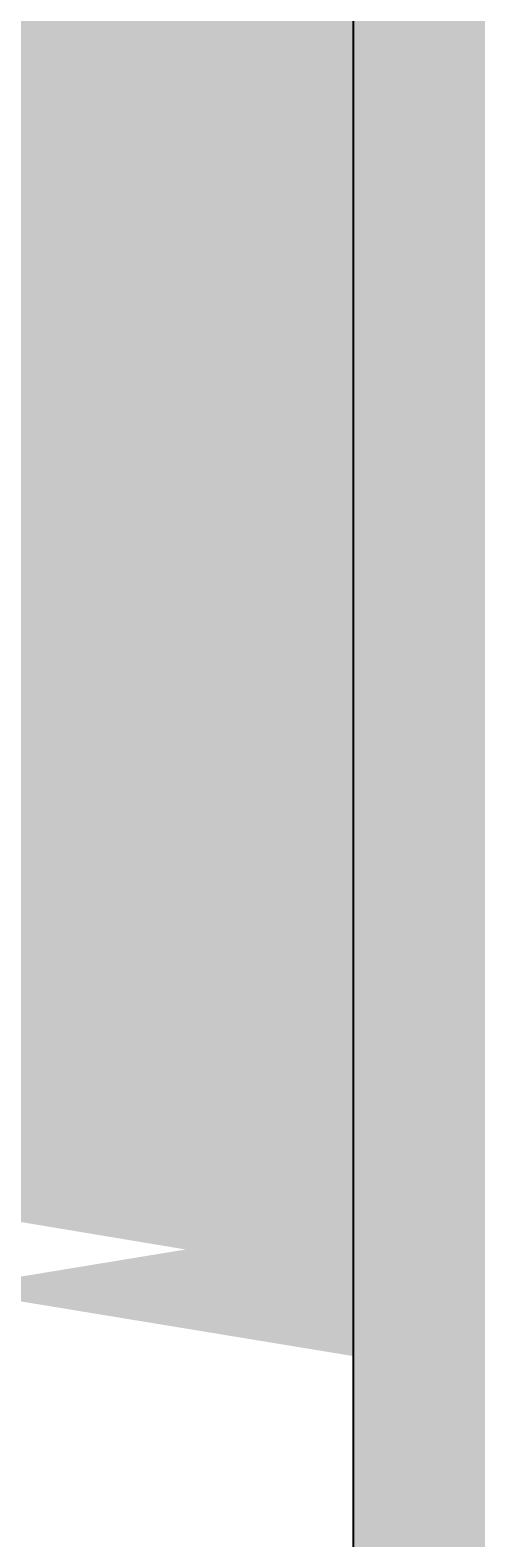
# Model space of a CAD drawing. Units: millimetres. Extents: x -22994 to 29398, y -19990 to 20176.
# Tile 42 of 135: x 190 to 198, y 54 to 78. Entities that reach past the tile are written whole.
import ezdxf
from ezdxf import colors
from ezdxf.entities.mleader import LeaderData, LeaderLine
from ezdxf.math import Vec2, Vec3

# ---------------------------------------------------------------- set-up
doc = ezdxf.new("R2010")
doc.units = ezdxf.units.MM
doc.header["$MEASUREMENT"] = 0
for name, color, linetype, lineweight in [('M-ANNO-TEXT', 7, 'Continuous', 25), ('M-DIMS', 2, 'Continuous', 18), ('M-EQPM', 7, 'Continuous', 25), ('M-EQPM-PATT', 7, 'Continuous', 18)]:
    doc.layers.add(name, color=color, linetype=linetype, lineweight=lineweight)
doc.styles.get("Standard").update_dxf_attribs({"font": 'arial.ttf'})
doc.dimstyles.get("Standard").update_dxf_attribs({"dimtxt": 0.18, "dimasz": 10000, "dimexe": 0.18, "dimexo": 0.0625, "dimgap": 0.09, "dimtad": 0, "dimtih": 1, "dimtoh": 1, "dimdec": 0, "dimzin": 0, "dimdsep": 46, "dimtxsty": 'Standard', "dimcen": 0.09, "dimadec": 0, "dimazin": 0, "dimtfac": 1, "dimtdec": 0, "dimtofl": 0, "dimtmove": 0, "dimatfit": 3, "dimfxl": 1, "dimtolj": 1, "dimtzin": 0, "dimlwd": 30, "dimarcsym": 0})

# ---------------------------------------------------------------- blocks, each defined once
blk = doc.blocks.new('*D2')
at = {"layer": 'Defpoints', "color": 0, "transparency": 16777216}
for p in [(6.677, 10.271), (290.852, 10.271), (290.852, -5.079)]:
    blk.add_point(p, dxfattribs=at)
at = {"layer": 'M-DIMS', "color": 0, "lineweight": -2, "transparency": 16777216}
for p, q in [((6.677, 10.209), (6.677, -5.259)), ((290.852, 10.209), (290.852, -5.259))]:
    blk.add_line(p, q, dxfattribs=at)
at = {"layer": 'M-DIMS', "color": 0, "lineweight": 30, "transparency": 16777216}
for p, q in [((-9993.323, -5.079), (-19993.323, -5.079)), ((10290.852, -5.079), (20290.852, -5.079))]:
    blk.add_line(p, q, dxfattribs=at)
at = {"layer": 'M-DIMS', "color": 0, "transparency": 16777216}
for points in [[(-9993.323, 1661.588), (-9993.323, -1671.745), (6.677, -5.079)], [(10290.852, 1661.588), (10290.852, -1671.745), (290.852, -5.079)]]:
    blk.add_solid(points, dxfattribs=at)
at = {"layer": 'M-DIMS', "color": 0, "transparency": 16777216, "insert": (148.765, -5.079), "char_height": 0.18, "attachment_point": 5}
blk.add_mtext('\\A1;284.2', dxfattribs=at)
blk = doc.blocks.new('*D3')
at = {"layer": 'Defpoints', "color": 0, "transparency": 16777216}
for p in [(110.265, 204.165), (110.265, 176.366), (95.833, 127.967)]:
    blk.add_point(p, dxfattribs=at)
at = {"layer": 'M-DIMS', "color": 0, "lineweight": -2, "transparency": 16777216}
for p, q in [((95.833, 128.03), (95.833, 204.345)), ((110.265, 176.429), (110.265, 204.345))]:
    blk.add_line(p, q, dxfattribs=at)
at = {"layer": 'M-DIMS', "color": 0, "lineweight": 30, "transparency": 16777216}
for p, q in [((-9904.167, 204.165), (-19904.167, 204.165)), ((10110.265, 204.165), (20110.265, 204.165))]:
    blk.add_line(p, q, dxfattribs=at)
at = {"layer": 'M-DIMS', "color": 0, "transparency": 16777216}
for points in [[(-9904.167, 1870.832), (-9904.167, -1462.501), (95.833, 204.165)], [(10110.265, 1870.832), (10110.265, -1462.501), (110.265, 204.165)]]:
    blk.add_solid(points, dxfattribs=at)
at = {"layer": 'M-DIMS', "color": 0, "transparency": 16777216, "insert": (103.049, 204.165), "char_height": 0.18, "attachment_point": 5}
blk.add_mtext('\\A1;14.432', dxfattribs=at)
blk = doc.blocks.new('*D4')
at = {"layer": 'Defpoints', "color": 0, "transparency": 16777216}
for p in [(116.265, 204.165), (110.265, 176.366), (116.265, 176.366)]:
    blk.add_point(p, dxfattribs=at)
at = {"layer": 'M-DIMS', "color": 0, "lineweight": -2, "transparency": 16777216}
for p, q in [((110.265, 176.429), (110.265, 204.345)), ((116.265, 176.429), (116.265, 204.345))]:
    blk.add_line(p, q, dxfattribs=at)
at = {"layer": 'M-DIMS', "color": 0, "lineweight": 30, "transparency": 16777216}
for p, q in [((-9889.735, 204.165), (-19889.735, 204.165)), ((10116.265, 204.165), (20116.265, 204.165))]:
    blk.add_line(p, q, dxfattribs=at)
at = {"layer": 'M-DIMS', "color": 0, "transparency": 16777216}
for points in [[(-9889.735, 1870.832), (-9889.735, -1462.501), (110.265, 204.165)], [(10116.265, 1870.832), (10116.265, -1462.501), (116.265, 204.165)]]:
    blk.add_solid(points, dxfattribs=at)
at = {"layer": 'M-DIMS', "color": 0, "transparency": 16777216, "insert": (113.265, 204.165), "char_height": 0.18, "attachment_point": 5}
blk.add_mtext('\\A1;6', dxfattribs=at)
blk = doc.blocks.new('*D5')
at = {"layer": 'Defpoints', "color": 0, "transparency": 16777216}
for p in [(181.265, 204.165), (116.265, 176.366), (181.265, 176.366)]:
    blk.add_point(p, dxfattribs=at)
at = {"layer": 'M-DIMS', "color": 0, "lineweight": -2, "transparency": 16777216}
for p, q in [((116.265, 176.429), (116.265, 204.345)), ((181.265, 176.429), (181.265, 204.345))]:
    blk.add_line(p, q, dxfattribs=at)
at = {"layer": 'M-DIMS', "color": 0, "lineweight": 30, "transparency": 16777216}
for p, q in [((-9883.735, 204.165), (-19883.735, 204.165)), ((10181.265, 204.165), (20181.265, 204.165))]:
    blk.add_line(p, q, dxfattribs=at)
at = {"layer": 'M-DIMS', "color": 0, "transparency": 16777216}
for points in [[(-9883.735, 1870.832), (-9883.735, -1462.501), (116.265, 204.165)], [(10181.265, 1870.832), (10181.265, -1462.501), (181.265, 204.165)]]:
    blk.add_solid(points, dxfattribs=at)
at = {"layer": 'M-DIMS', "color": 0, "transparency": 16777216, "insert": (148.765, 204.165), "char_height": 0.18, "attachment_point": 5}
blk.add_mtext('\\A1;65', dxfattribs=at)
blk = doc.blocks.new('*D6')
at = {"layer": 'Defpoints', "color": 0, "transparency": 16777216}
for p in [(187.265, 204.165), (181.265, 176.366), (187.265, 176.366)]:
    blk.add_point(p, dxfattribs=at)
at = {"layer": 'M-DIMS', "color": 0, "lineweight": -2, "transparency": 16777216}
for p, q in [((181.265, 176.429), (181.265, 204.345)), ((187.265, 176.429), (187.265, 204.345))]:
    blk.add_line(p, q, dxfattribs=at)
at = {"layer": 'M-DIMS', "color": 0, "lineweight": 30, "transparency": 16777216}
for p, q in [((-9818.735, 204.165), (-19818.735, 204.165)), ((10187.265, 204.165), (20187.265, 204.165))]:
    blk.add_line(p, q, dxfattribs=at)
at = {"layer": 'M-DIMS', "color": 0, "transparency": 16777216}
for points in [[(-9818.735, 1870.832), (-9818.735, -1462.501), (181.265, 204.165)], [(10187.265, 1870.832), (10187.265, -1462.501), (187.265, 204.165)]]:
    blk.add_solid(points, dxfattribs=at)
at = {"layer": 'M-DIMS', "color": 0, "transparency": 16777216, "insert": (184.265, 204.165), "char_height": 0.18, "attachment_point": 5}
blk.add_mtext('\\A1;6', dxfattribs=at)
blk = doc.blocks.new('*D7')
at = {"layer": 'Defpoints', "color": 0, "transparency": 16777216}
for p in [(201.697, 204.165), (187.265, 176.366), (201.697, 127.967)]:
    blk.add_point(p, dxfattribs=at)
at = {"layer": 'M-DIMS', "color": 0, "lineweight": -2, "transparency": 16777216}
for p, q in [((187.265, 176.429), (187.265, 204.345)), ((201.697, 128.03), (201.697, 204.345))]:
    blk.add_line(p, q, dxfattribs=at)
at = {"layer": 'M-DIMS', "color": 0, "lineweight": 30, "transparency": 16777216}
for p, q in [((-9812.735, 204.165), (-19812.735, 204.165)), ((10201.697, 204.165), (20201.697, 204.165))]:
    blk.add_line(p, q, dxfattribs=at)
at = {"layer": 'M-DIMS', "color": 0, "transparency": 16777216}
for points in [[(-9812.735, 1870.832), (-9812.735, -1462.501), (187.265, 204.165)], [(10201.697, 1870.832), (10201.697, -1462.501), (201.697, 204.165)]]:
    blk.add_solid(points, dxfattribs=at)
at = {"layer": 'M-DIMS', "color": 0, "transparency": 16777216, "insert": (194.481, 204.165), "char_height": 0.18, "attachment_point": 5}
blk.add_mtext('\\A1;14.432', dxfattribs=at)
blk = doc.blocks.new('*D8')
at = {"layer": 'Defpoints', "color": 0, "transparency": 16777216}
for p in [(227.648, 204.165), (227.648, 146.73), (201.697, 127.967)]:
    blk.add_point(p, dxfattribs=at)
at = {"layer": 'M-DIMS', "color": 0, "lineweight": -2, "transparency": 16777216}
for p, q in [((201.697, 128.03), (201.697, 204.345)), ((227.648, 146.792), (227.648, 204.345))]:
    blk.add_line(p, q, dxfattribs=at)
at = {"layer": 'M-DIMS', "color": 0, "lineweight": 30, "transparency": 16777216}
for p, q in [((-9798.303, 204.165), (-19798.303, 204.165)), ((10227.648, 204.165), (20227.648, 204.165))]:
    blk.add_line(p, q, dxfattribs=at)
at = {"layer": 'M-DIMS', "color": 0, "transparency": 16777216}
for points in [[(-9798.303, 1870.832), (-9798.303, -1462.501), (201.697, 204.165)], [(10227.648, 1870.832), (10227.648, -1462.501), (227.648, 204.165)]]:
    blk.add_solid(points, dxfattribs=at)
at = {"layer": 'M-DIMS', "color": 0, "transparency": 16777216, "insert": (214.673, 204.165), "char_height": 0.18, "attachment_point": 5}
blk.add_mtext('\\A1;25.95', dxfattribs=at)
blk = doc.blocks.new('*D9')
at = {"layer": 'Defpoints', "color": 0, "transparency": 16777216}
for p in [(187.265, 176.366), (306.202, 176.366), (290.852, 10.271)]:
    blk.add_point(p, dxfattribs=at)
at = {"layer": 'M-DIMS', "color": 0, "lineweight": 30, "transparency": 16777216}
for p, q in [((306.202, 10176.366), (306.202, 20176.366)), ((306.202, -9989.729), (306.202, -19989.729))]:
    blk.add_line(p, q, dxfattribs=at)
at = {"layer": 'M-DIMS', "color": 0, "lineweight": -2, "transparency": 16777216}
for p, q in [((187.327, 176.366), (306.382, 176.366)), ((290.915, 10.271), (306.382, 10.271))]:
    blk.add_line(p, q, dxfattribs=at)
at = {"layer": 'M-DIMS', "color": 0, "transparency": 16777216}
for points in [[(-1360.465, 10176.366), (1972.869, 10176.366), (306.202, 176.366)], [(-1360.465, -9989.729), (1972.869, -9989.729), (306.202, 10.271)]]:
    blk.add_solid(points, dxfattribs=at)
at = {"layer": 'M-DIMS', "color": 0, "transparency": 16777216, "insert": (306.202, 93.319), "char_height": 0.18, "attachment_point": 5}
blk.add_mtext('\\A1;166.1', dxfattribs=at)
blk = doc.blocks.new('*D10')
at = {"layer": 'Defpoints', "color": 0, "transparency": 16777216}
for p in [(125.65, 136.071), (133.346, 136.071), (133.346, -5.079)]:
    blk.add_point(p, dxfattribs=at)
at = {"layer": 'M-DIMS', "color": 0, "lineweight": -2, "transparency": 16777216}
for p, q in [((125.65, 136.009), (125.65, -5.259)), ((133.346, 136.009), (133.346, -5.259))]:
    blk.add_line(p, q, dxfattribs=at)
at = {"layer": 'M-DIMS', "color": 0, "lineweight": 30, "transparency": 16777216}
for p, q in [((-9874.35, -5.079), (-19874.35, -5.079)), ((10133.346, -5.079), (20133.346, -5.079))]:
    blk.add_line(p, q, dxfattribs=at)
at = {"layer": 'M-DIMS', "color": 0, "transparency": 16777216}
for points in [[(-9874.35, 1661.588), (-9874.35, -1671.745), (125.65, -5.079)], [(10133.346, 1661.588), (10133.346, -1671.745), (133.346, -5.079)]]:
    blk.add_solid(points, dxfattribs=at)
at = {"layer": 'M-DIMS', "color": 0, "transparency": 16777216, "insert": (129.498, -5.079), "char_height": 0.18, "attachment_point": 5}
blk.add_mtext('\\A1;7.696', dxfattribs=at)
blk = doc.blocks.new('*D11')
at = {"layer": 'Defpoints', "color": 0, "transparency": 16777216}
for p in [(133.346, 136.071), (135.65, 136.071), (135.65, -5.079)]:
    blk.add_point(p, dxfattribs=at)
at = {"layer": 'M-DIMS', "color": 0, "lineweight": -2, "transparency": 16777216}
for p, q in [((133.346, 136.009), (133.346, -5.259)), ((135.65, 136.009), (135.65, -5.259))]:
    blk.add_line(p, q, dxfattribs=at)
at = {"layer": 'M-DIMS', "color": 0, "lineweight": 30, "transparency": 16777216}
for p, q in [((-9866.654, -5.079), (-19866.654, -5.079)), ((10135.65, -5.079), (20135.65, -5.079))]:
    blk.add_line(p, q, dxfattribs=at)
at = {"layer": 'M-DIMS', "color": 0, "transparency": 16777216}
for points in [[(-9866.654, 1661.588), (-9866.654, -1671.745), (133.346, -5.079)], [(10135.65, 1661.588), (10135.65, -1671.745), (135.65, -5.079)]]:
    blk.add_solid(points, dxfattribs=at)
at = {"layer": 'M-DIMS', "color": 0, "transparency": 16777216, "insert": (134.498, -5.079), "char_height": 0.18, "attachment_point": 5}
blk.add_mtext('\\A1;2.304', dxfattribs=at)
blk = doc.blocks.new('*D12')
at = {"layer": 'Defpoints', "color": 0, "transparency": 16777216}
for p in [(135.65, 136.071), (145.65, 136.071), (145.65, -5.079)]:
    blk.add_point(p, dxfattribs=at)
at = {"layer": 'M-DIMS', "color": 0, "lineweight": -2, "transparency": 16777216}
for p, q in [((135.65, 136.009), (135.65, -5.259)), ((145.65, 136.009), (145.65, -5.259))]:
    blk.add_line(p, q, dxfattribs=at)
at = {"layer": 'M-DIMS', "color": 0, "lineweight": 30, "transparency": 16777216}
for p, q in [((-9864.35, -5.079), (-19864.35, -5.079)), ((10145.65, -5.079), (20145.65, -5.079))]:
    blk.add_line(p, q, dxfattribs=at)
at = {"layer": 'M-DIMS', "color": 0, "transparency": 16777216}
for points in [[(-9864.35, 1661.588), (-9864.35, -1671.745), (135.65, -5.079)], [(10145.65, 1661.588), (10145.65, -1671.745), (145.65, -5.079)]]:
    blk.add_solid(points, dxfattribs=at)
at = {"layer": 'M-DIMS', "color": 0, "transparency": 16777216, "insert": (140.65, -5.079), "char_height": 0.18, "attachment_point": 5}
blk.add_mtext('\\A1;10', dxfattribs=at)
blk = doc.blocks.new('*D13')
at = {"layer": 'Defpoints', "color": 0, "transparency": 16777216}
for p in [(145.65, 136.071), (155.65, 136.071), (155.65, -5.079)]:
    blk.add_point(p, dxfattribs=at)
at = {"layer": 'M-DIMS', "color": 0, "lineweight": -2, "transparency": 16777216}
for p, q in [((145.65, 136.009), (145.65, -5.259)), ((155.65, 136.009), (155.65, -5.259))]:
    blk.add_line(p, q, dxfattribs=at)
at = {"layer": 'M-DIMS', "color": 0, "lineweight": 30, "transparency": 16777216}
for p, q in [((-9854.35, -5.079), (-19854.35, -5.079)), ((10155.65, -5.079), (20155.65, -5.079))]:
    blk.add_line(p, q, dxfattribs=at)
at = {"layer": 'M-DIMS', "color": 0, "transparency": 16777216}
for points in [[(-9854.35, 1661.588), (-9854.35, -1671.745), (145.65, -5.079)], [(10155.65, 1661.588), (10155.65, -1671.745), (155.65, -5.079)]]:
    blk.add_solid(points, dxfattribs=at)
at = {"layer": 'M-DIMS', "color": 0, "transparency": 16777216, "insert": (150.65, -5.079), "char_height": 0.18, "attachment_point": 5}
blk.add_mtext('\\A1;10', dxfattribs=at)
blk = doc.blocks.new('*D14')
at = {"layer": 'Defpoints', "color": 0, "transparency": 16777216}
for p in [(155.65, 136.071), (165.65, 136.071), (165.65, -5.079)]:
    blk.add_point(p, dxfattribs=at)
at = {"layer": 'M-DIMS', "color": 0, "lineweight": -2, "transparency": 16777216}
for p, q in [((155.65, 136.009), (155.65, -5.259)), ((165.65, 136.009), (165.65, -5.259))]:
    blk.add_line(p, q, dxfattribs=at)
at = {"layer": 'M-DIMS', "color": 0, "lineweight": 30, "transparency": 16777216}
for p, q in [((-9844.35, -5.079), (-19844.35, -5.079)), ((10165.65, -5.079), (20165.65, -5.079))]:
    blk.add_line(p, q, dxfattribs=at)
at = {"layer": 'M-DIMS', "color": 0, "transparency": 16777216}
for points in [[(-9844.35, 1661.588), (-9844.35, -1671.745), (155.65, -5.079)], [(10165.65, 1661.588), (10165.65, -1671.745), (165.65, -5.079)]]:
    blk.add_solid(points, dxfattribs=at)
at = {"layer": 'M-DIMS', "color": 0, "transparency": 16777216, "insert": (160.65, -5.079), "char_height": 0.18, "attachment_point": 5}
blk.add_mtext('\\A1;10', dxfattribs=at)
blk = doc.blocks.new('*D15')
at = {"layer": 'Defpoints', "color": 0, "transparency": 16777216}
for p in [(173.346, 154.788), (173.346, 136.071), (306.202, 136.071)]:
    blk.add_point(p, dxfattribs=at)
at = {"layer": 'M-DIMS', "color": 0, "lineweight": 30, "transparency": 16777216}
for p, q in [((306.202, 10154.788), (306.202, 20154.788)), ((306.202, -9863.929), (306.202, -19863.929))]:
    blk.add_line(p, q, dxfattribs=at)
at = {"layer": 'M-DIMS', "color": 0, "lineweight": -2, "transparency": 16777216}
for p, q in [((173.408, 154.788), (306.382, 154.788)), ((173.408, 136.071), (306.382, 136.071))]:
    blk.add_line(p, q, dxfattribs=at)
at = {"layer": 'M-DIMS', "color": 0, "transparency": 16777216}
for points in [[(-1360.465, 10154.788), (1972.869, 10154.788), (306.202, 154.788)], [(-1360.465, -9863.929), (1972.869, -9863.929), (306.202, 136.071)]]:
    blk.add_solid(points, dxfattribs=at)
at = {"layer": 'M-DIMS', "color": 0, "transparency": 16777216, "insert": (306.202, 145.43), "char_height": 0.18, "attachment_point": 5}
blk.add_mtext('\\A1;18.717', dxfattribs=at)
blk = doc.blocks.new('*D16')
at = {"layer": 'Defpoints', "color": 0, "transparency": 16777216}
for p in [(120.17, 204.165), (110.466, 48.035), (120.17, 48.035)]:
    blk.add_point(p, dxfattribs=at)
at = {"layer": 'M-DIMS', "color": 0, "lineweight": -2, "transparency": 16777216}
for p, q in [((110.466, 48.097), (110.466, 204.345)), ((120.17, 48.097), (120.17, 204.345))]:
    blk.add_line(p, q, dxfattribs=at)
at = {"layer": 'M-DIMS', "color": 0, "lineweight": 30, "transparency": 16777216}
for p, q in [((-9889.534, 204.165), (-19889.534, 204.165)), ((10120.17, 204.165), (20120.17, 204.165))]:
    blk.add_line(p, q, dxfattribs=at)
at = {"layer": 'M-DIMS', "color": 0, "transparency": 16777216}
for points in [[(-9889.534, 1870.832), (-9889.534, -1462.501), (110.466, 204.165)], [(10120.17, 1870.832), (10120.17, -1462.501), (120.17, 204.165)]]:
    blk.add_solid(points, dxfattribs=at)
at = {"layer": 'M-DIMS', "color": 0, "transparency": 16777216, "insert": (115.318, 204.165), "char_height": 0.18, "attachment_point": 5}
blk.add_mtext('\\A1;9.704', dxfattribs=at)
blk = doc.blocks.new('*D17')
at = {"layer": 'Defpoints', "color": 0, "transparency": 16777216}
for p in [(126.17, 204.165), (120.17, 48.035), (126.17, 48.035)]:
    blk.add_point(p, dxfattribs=at)
at = {"layer": 'M-DIMS', "color": 0, "lineweight": -2, "transparency": 16777216}
for p, q in [((120.17, 48.097), (120.17, 204.345)), ((126.17, 48.097), (126.17, 204.345))]:
    blk.add_line(p, q, dxfattribs=at)
at = {"layer": 'M-DIMS', "color": 0, "lineweight": 30, "transparency": 16777216}
for p, q in [((-9879.83, 204.165), (-19879.83, 204.165)), ((10126.17, 204.165), (20126.17, 204.165))]:
    blk.add_line(p, q, dxfattribs=at)
at = {"layer": 'M-DIMS', "color": 0, "transparency": 16777216}
for points in [[(-9879.83, 1870.832), (-9879.83, -1462.501), (120.17, 204.165)], [(10126.17, 1870.832), (10126.17, -1462.501), (126.17, 204.165)]]:
    blk.add_solid(points, dxfattribs=at)
at = {"layer": 'M-DIMS', "color": 0, "transparency": 16777216, "insert": (123.17, 204.165), "char_height": 0.18, "attachment_point": 5}
blk.add_mtext('\\A1;6', dxfattribs=at)
blk = doc.blocks.new('*D18')
at = {"layer": 'Defpoints', "color": 0, "transparency": 16777216}
for p in [(132.17, 204.165), (126.17, 48.035), (132.17, 48.035)]:
    blk.add_point(p, dxfattribs=at)
at = {"layer": 'M-DIMS', "color": 0, "lineweight": -2, "transparency": 16777216}
for p, q in [((126.17, 48.097), (126.17, 204.345)), ((132.17, 48.097), (132.17, 204.345))]:
    blk.add_line(p, q, dxfattribs=at)
at = {"layer": 'M-DIMS', "color": 0, "lineweight": 30, "transparency": 16777216}
for p, q in [((-9873.83, 204.165), (-19873.83, 204.165)), ((10132.17, 204.165), (20132.17, 204.165))]:
    blk.add_line(p, q, dxfattribs=at)
at = {"layer": 'M-DIMS', "color": 0, "transparency": 16777216}
for points in [[(-9873.83, 1870.832), (-9873.83, -1462.501), (126.17, 204.165)], [(10132.17, 1870.832), (10132.17, -1462.501), (132.17, 204.165)]]:
    blk.add_solid(points, dxfattribs=at)
at = {"layer": 'M-DIMS', "color": 0, "transparency": 16777216, "insert": (129.17, 204.165), "char_height": 0.18, "attachment_point": 5}
blk.add_mtext('\\A1;6', dxfattribs=at)
blk = doc.blocks.new('*D19')
at = {"layer": 'Defpoints', "color": 0, "transparency": 16777216}
for p in [(138.17, 204.165), (132.17, 48.035), (138.17, 48.035)]:
    blk.add_point(p, dxfattribs=at)
at = {"layer": 'M-DIMS', "color": 0, "lineweight": -2, "transparency": 16777216}
for p, q in [((132.17, 48.097), (132.17, 204.345)), ((138.17, 48.097), (138.17, 204.345))]:
    blk.add_line(p, q, dxfattribs=at)
at = {"layer": 'M-DIMS', "color": 0, "lineweight": 30, "transparency": 16777216}
for p, q in [((-9867.83, 204.165), (-19867.83, 204.165)), ((10138.17, 204.165), (20138.17, 204.165))]:
    blk.add_line(p, q, dxfattribs=at)
at = {"layer": 'M-DIMS', "color": 0, "transparency": 16777216}
for points in [[(-9867.83, 1870.832), (-9867.83, -1462.501), (132.17, 204.165)], [(10138.17, 1870.832), (10138.17, -1462.501), (138.17, 204.165)]]:
    blk.add_solid(points, dxfattribs=at)
at = {"layer": 'M-DIMS', "color": 0, "transparency": 16777216, "insert": (135.17, 204.165), "char_height": 0.18, "attachment_point": 5}
blk.add_mtext('\\A1;6', dxfattribs=at)
blk = doc.blocks.new('*D20')
at = {"layer": 'Defpoints', "color": 0, "transparency": 16777216}
for p in [(144.17, 204.165), (138.17, 48.035), (144.17, 48.035)]:
    blk.add_point(p, dxfattribs=at)
at = {"layer": 'M-DIMS', "color": 0, "lineweight": -2, "transparency": 16777216}
for p, q in [((138.17, 48.097), (138.17, 204.345)), ((144.17, 48.097), (144.17, 204.345))]:
    blk.add_line(p, q, dxfattribs=at)
at = {"layer": 'M-DIMS', "color": 0, "lineweight": 30, "transparency": 16777216}
for p, q in [((-9861.83, 204.165), (-19861.83, 204.165)), ((10144.17, 204.165), (20144.17, 204.165))]:
    blk.add_line(p, q, dxfattribs=at)
at = {"layer": 'M-DIMS', "color": 0, "transparency": 16777216}
for points in [[(-9861.83, 1870.832), (-9861.83, -1462.501), (138.17, 204.165)], [(10144.17, 1870.832), (10144.17, -1462.501), (144.17, 204.165)]]:
    blk.add_solid(points, dxfattribs=at)
at = {"layer": 'M-DIMS', "color": 0, "transparency": 16777216, "insert": (141.17, 204.165), "char_height": 0.18, "attachment_point": 5}
blk.add_mtext('\\A1;6', dxfattribs=at)
blk = doc.blocks.new('*D21')
at = {"layer": 'Defpoints', "color": 0, "transparency": 16777216}
for p in [(149.116, 204.165), (144.17, 48.035), (149.116, 48.035)]:
    blk.add_point(p, dxfattribs=at)
at = {"layer": 'M-DIMS', "color": 0, "lineweight": -2, "transparency": 16777216}
for p, q in [((144.17, 48.097), (144.17, 204.345)), ((149.116, 48.097), (149.116, 204.345))]:
    blk.add_line(p, q, dxfattribs=at)
at = {"layer": 'M-DIMS', "color": 0, "lineweight": 30, "transparency": 16777216}
for p, q in [((-9855.83, 204.165), (-19855.83, 204.165)), ((10149.116, 204.165), (20149.116, 204.165))]:
    blk.add_line(p, q, dxfattribs=at)
at = {"layer": 'M-DIMS', "color": 0, "transparency": 16777216}
for points in [[(-9855.83, 1870.832), (-9855.83, -1462.501), (144.17, 204.165)], [(10149.116, 1870.832), (10149.116, -1462.501), (149.116, 204.165)]]:
    blk.add_solid(points, dxfattribs=at)
at = {"layer": 'M-DIMS', "color": 0, "transparency": 16777216, "insert": (146.643, 204.165), "char_height": 0.18, "attachment_point": 5}
blk.add_mtext('\\A1;4.945', dxfattribs=at)
blk = doc.blocks.new('*D22')
at = {"layer": 'Defpoints', "color": 0, "transparency": 16777216}
for p in [(149.116, 30.99), (155.116, 30.99), (155.116, -5.079)]:
    blk.add_point(p, dxfattribs=at)
at = {"layer": 'M-DIMS', "color": 0, "lineweight": -2, "transparency": 16777216}
for p, q in [((149.116, 30.927), (149.116, -5.259)), ((155.116, 30.927), (155.116, -5.259))]:
    blk.add_line(p, q, dxfattribs=at)
at = {"layer": 'M-DIMS', "color": 0, "lineweight": 30, "transparency": 16777216}
for p, q in [((-9850.884, -5.079), (-19850.884, -5.079)), ((10155.116, -5.079), (20155.116, -5.079))]:
    blk.add_line(p, q, dxfattribs=at)
at = {"layer": 'M-DIMS', "color": 0, "transparency": 16777216}
for points in [[(-9850.884, 1661.588), (-9850.884, -1671.745), (149.116, -5.079)], [(10155.116, 1661.588), (10155.116, -1671.745), (155.116, -5.079)]]:
    blk.add_solid(points, dxfattribs=at)
at = {"layer": 'M-DIMS', "color": 0, "transparency": 16777216, "insert": (152.116, -5.079), "char_height": 0.18, "attachment_point": 5}
blk.add_mtext('\\A1;6', dxfattribs=at)
blk = doc.blocks.new('*D23')
at = {"layer": 'Defpoints', "color": 0, "transparency": 16777216}
for p in [(155.116, 30.99), (161.116, 30.99), (161.116, -5.079)]:
    blk.add_point(p, dxfattribs=at)
at = {"layer": 'M-DIMS', "color": 0, "lineweight": -2, "transparency": 16777216}
for p, q in [((155.116, 30.927), (155.116, -5.259)), ((161.116, 30.927), (161.116, -5.259))]:
    blk.add_line(p, q, dxfattribs=at)
at = {"layer": 'M-DIMS', "color": 0, "lineweight": 30, "transparency": 16777216}
for p, q in [((-9844.884, -5.079), (-19844.884, -5.079)), ((10161.116, -5.079), (20161.116, -5.079))]:
    blk.add_line(p, q, dxfattribs=at)
at = {"layer": 'M-DIMS', "color": 0, "transparency": 16777216}
for points in [[(-9844.884, 1661.588), (-9844.884, -1671.745), (155.116, -5.079)], [(10161.116, 1661.588), (10161.116, -1671.745), (161.116, -5.079)]]:
    blk.add_solid(points, dxfattribs=at)
at = {"layer": 'M-DIMS', "color": 0, "transparency": 16777216, "insert": (158.116, -5.079), "char_height": 0.18, "attachment_point": 5}
blk.add_mtext('\\A1;6', dxfattribs=at)
blk = doc.blocks.new('*D24')
at = {"layer": 'Defpoints', "color": 0, "transparency": 16777216}
for p in [(161.116, 30.99), (166.439, 30.99), (166.439, -5.079)]:
    blk.add_point(p, dxfattribs=at)
at = {"layer": 'M-DIMS', "color": 0, "lineweight": -2, "transparency": 16777216}
for p, q in [((161.116, 30.927), (161.116, -5.259)), ((166.439, 30.927), (166.439, -5.259))]:
    blk.add_line(p, q, dxfattribs=at)
at = {"layer": 'M-DIMS', "color": 0, "lineweight": 30, "transparency": 16777216}
for p, q in [((-9838.884, -5.079), (-19838.884, -5.079)), ((10166.439, -5.079), (20166.439, -5.079))]:
    blk.add_line(p, q, dxfattribs=at)
at = {"layer": 'M-DIMS', "color": 0, "transparency": 16777216}
for points in [[(-9838.884, 1661.588), (-9838.884, -1671.745), (161.116, -5.079)], [(10166.439, 1661.588), (10166.439, -1671.745), (166.439, -5.079)]]:
    blk.add_solid(points, dxfattribs=at)
at = {"layer": 'M-DIMS', "color": 0, "transparency": 16777216, "insert": (163.777, -5.079), "char_height": 0.18, "attachment_point": 5}
blk.add_mtext('\\A1;5.323', dxfattribs=at)
blk = doc.blocks.new('*D25')
at = {"layer": 'Defpoints', "color": 0, "transparency": 16777216}
for p in [(166.439, 30.99), (172.439, 30.99), (172.439, -5.079)]:
    blk.add_point(p, dxfattribs=at)
at = {"layer": 'M-DIMS', "color": 0, "lineweight": -2, "transparency": 16777216}
for p, q in [((166.439, 30.927), (166.439, -5.259)), ((172.439, 30.927), (172.439, -5.259))]:
    blk.add_line(p, q, dxfattribs=at)
at = {"layer": 'M-DIMS', "color": 0, "lineweight": 30, "transparency": 16777216}
for p, q in [((-9833.561, -5.079), (-19833.561, -5.079)), ((10172.439, -5.079), (20172.439, -5.079))]:
    blk.add_line(p, q, dxfattribs=at)
at = {"layer": 'M-DIMS', "color": 0, "transparency": 16777216}
for points in [[(-9833.561, 1661.588), (-9833.561, -1671.745), (166.439, -5.079)], [(10172.439, 1661.588), (10172.439, -1671.745), (172.439, -5.079)]]:
    blk.add_solid(points, dxfattribs=at)
at = {"layer": 'M-DIMS', "color": 0, "transparency": 16777216, "insert": (169.439, -5.079), "char_height": 0.18, "attachment_point": 5}
blk.add_mtext('\\A1;6', dxfattribs=at)
blk = doc.blocks.new('*D26')
at = {"layer": 'Defpoints', "color": 0, "transparency": 16777216}
for p in [(172.439, 30.99), (178.439, 30.99), (178.439, -5.079)]:
    blk.add_point(p, dxfattribs=at)
at = {"layer": 'M-DIMS', "color": 0, "lineweight": -2, "transparency": 16777216}
for p, q in [((172.439, 30.927), (172.439, -5.259)), ((178.439, 30.927), (178.439, -5.259))]:
    blk.add_line(p, q, dxfattribs=at)
at = {"layer": 'M-DIMS', "color": 0, "lineweight": 30, "transparency": 16777216}
for p, q in [((-9827.561, -5.079), (-19827.561, -5.079)), ((10178.439, -5.079), (20178.439, -5.079))]:
    blk.add_line(p, q, dxfattribs=at)
at = {"layer": 'M-DIMS', "color": 0, "transparency": 16777216}
for points in [[(-9827.561, 1661.588), (-9827.561, -1671.745), (172.439, -5.079)], [(10178.439, 1661.588), (10178.439, -1671.745), (178.439, -5.079)]]:
    blk.add_solid(points, dxfattribs=at)
at = {"layer": 'M-DIMS', "color": 0, "transparency": 16777216, "insert": (175.439, -5.079), "char_height": 0.18, "attachment_point": 5}
blk.add_mtext('\\A1;6', dxfattribs=at)
blk = doc.blocks.new('*D27')
at = {"layer": 'Defpoints', "color": 0, "transparency": 16777216}
for p in [(178.439, 30.99), (188.117, 30.99), (188.117, -5.079)]:
    blk.add_point(p, dxfattribs=at)
at = {"layer": 'M-DIMS', "color": 0, "lineweight": -2, "transparency": 16777216}
for p, q in [((178.439, 30.927), (178.439, -5.259)), ((188.117, 30.927), (188.117, -5.259))]:
    blk.add_line(p, q, dxfattribs=at)
at = {"layer": 'M-DIMS', "color": 0, "lineweight": 30, "transparency": 16777216}
for p, q in [((-9821.561, -5.079), (-19821.561, -5.079)), ((10188.117, -5.079), (20188.117, -5.079))]:
    blk.add_line(p, q, dxfattribs=at)
at = {"layer": 'M-DIMS', "color": 0, "transparency": 16777216}
for points in [[(-9821.561, 1661.588), (-9821.561, -1671.745), (178.439, -5.079)], [(10188.117, 1661.588), (10188.117, -1671.745), (188.117, -5.079)]]:
    blk.add_solid(points, dxfattribs=at)
at = {"layer": 'M-DIMS', "color": 0, "transparency": 16777216, "insert": (183.278, -5.079), "char_height": 0.18, "attachment_point": 5}
blk.add_mtext('\\A1;9.679', dxfattribs=at)
blk = doc.blocks.new('*D28')
at = {"layer": 'Defpoints', "color": 0, "transparency": 16777216}
for p in [(188.117, 48.035), (306.202, 48.035), (188.117, 30.99)]:
    blk.add_point(p, dxfattribs=at)
at = {"layer": 'M-DIMS', "color": 0, "lineweight": 30, "transparency": 16777216}
for p, q in [((306.202, 10048.035), (306.202, 20048.035)), ((306.202, -9969.01), (306.202, -19969.01))]:
    blk.add_line(p, q, dxfattribs=at)
at = {"layer": 'M-DIMS', "color": 0, "lineweight": -2, "transparency": 16777216}
for p, q in [((188.18, 48.035), (306.382, 48.035)), ((188.18, 30.99), (306.382, 30.99))]:
    blk.add_line(p, q, dxfattribs=at)
at = {"layer": 'M-DIMS', "color": 0, "transparency": 16777216}
for points in [[(-1360.465, 10048.035), (1972.869, 10048.035), (306.202, 48.035)], [(-1360.465, -9969.01), (1972.869, -9969.01), (306.202, 30.99)]]:
    blk.add_solid(points, dxfattribs=at)
at = {"layer": 'M-DIMS', "color": 0, "transparency": 16777216, "insert": (306.202, 39.512), "char_height": 0.18, "attachment_point": 5}
blk.add_mtext('\\A1;17.045', dxfattribs=at)
blk = doc.blocks.new('*D29')
at = {"layer": 'Defpoints', "color": 0, "transparency": 16777216}
for p in [(36.801, 80.045), (64.03, 80.045)]:
    blk.add_point(p, dxfattribs=at)
at = {"layer": 'M-DIMS', "color": 0, "lineweight": -2, "transparency": 16777216}
for p, q in [((50.325, 80.045), (50.505, 80.045)), ((50.415, 79.955), (50.415, 80.135))]:
    blk.add_line(p, q, dxfattribs=at)
at = {"layer": 'M-DIMS', "color": 0, "lineweight": 30, "transparency": 16777216}
blk.add_line((20064.03, 80.03), (10064.03, 80.038), dxfattribs=at)
at = {"layer": 'M-DIMS', "color": 0, "transparency": 16777216}
blk.add_solid([(10064.031, 1746.704), (10064.028, -1586.629), (64.03, 80.045)], dxfattribs=at)
at = {"layer": 'M-DIMS', "color": 0, "transparency": 16777216, "insert": (20064.521, 80.03), "char_height": 0.18, "attachment_point": 5}
blk.add_mtext('\\A1;∅27.23', dxfattribs=at)
blk = doc.blocks.new('*D36')
at = {"layer": 'Defpoints', "color": 0, "transparency": 16777216}
for p in [(46.39, 31.303), (46.387, 26.593)]:
    blk.add_point(p, dxfattribs=at)
at = {"layer": 'M-DIMS', "color": 0, "lineweight": 30, "transparency": 16777216}
for p, q in [((57.15, 20031.301), (51.77, 10031.302)), ((10057.15, 20031.301), (57.15, 20031.301))]:
    blk.add_line(p, q, dxfattribs=at)
at = {"layer": 'M-DIMS', "color": 0, "lineweight": -2, "transparency": 16777216}
for p, q in [((46.299, 28.948), (46.479, 28.948)), ((46.389, 28.858), (46.389, 29.038))]:
    blk.add_line(p, q, dxfattribs=at)
at = {"layer": 'M-DIMS', "color": 0, "transparency": 16777216}
blk.add_solid([(-1614.896, 10032.199), (1718.436, 10030.405), (46.39, 31.303)], dxfattribs=at)
at = {"layer": 'M-DIMS', "color": 0, "transparency": 16777216, "insert": (10057.554, 20031.301), "char_height": 0.18, "attachment_point": 5}
blk.add_mtext('\\A1;∅4.71', dxfattribs=at)
blk = doc.blocks.new('*D37')
at = {"layer": 'Defpoints', "color": 0, "transparency": 16777216}
for p in [(54.834, 118.615), (59.494, 118.614)]:
    blk.add_point(p, dxfattribs=at)
at = {"layer": 'M-DIMS', "color": 0, "lineweight": -2, "transparency": 16777216}
for p, q in [((57.074, 118.614), (57.254, 118.614)), ((57.164, 118.524), (57.164, 118.704))]:
    blk.add_line(p, q, dxfattribs=at)
at = {"layer": 'M-DIMS', "color": 0, "lineweight": 30, "transparency": 16777216}
blk.add_line((20059.493, 116.253), (10059.494, 117.434), dxfattribs=at)
at = {"layer": 'M-DIMS', "color": 0, "transparency": 16777216}
blk.add_solid([(10059.69, 1784.1), (10059.297, -1549.233), (59.494, 118.614)], dxfattribs=at)
at = {"layer": 'M-DIMS', "color": 0, "transparency": 16777216, "insert": (20059.985, 116.253), "char_height": 0.18, "attachment_point": 5}
blk.add_mtext('\\A1;∅4.659', dxfattribs=at)

msp = doc.modelspace()

# ---------------------------------------------------------------- hatches: boundary and pattern name
at = {"layer": 'M-EQPM-PATT'}
h = msp.add_hatch(color=256, dxfattribs=at)
h.set_gradient(color1=(205, 32, 39), color2=(205, 32, 39), tint=1)
h.paths.add_polyline_path([(116.2647, 150.3662), (116.2647, 170.3662), (116.2647, 176.3662), (110.2647, 176.3662), (110.2647, 152.0276), (95.8327, 127.967), (95.8327, 16.6063), (201.6967, 16.6063), (201.6967, 127.967), (187.2647, 152.0276), (187.2647, 176.3662), (181.2647, 176.3662), (181.2647, 170.3662), (181.2647, 150.3662), (195.6967, 126.3055), (195.6967, 22.6063), (101.8327, 22.6063), (101.8327, 126.3055)])
h.paths.add_polyline_path([(185.2208, 88.6347), (101.8327, 88.6347), (101.8327, 87.6347), (182.8066, 87.6347), (178.7313, 83.5594), (195.6967, 83.5594), (195.6967, 84.5594), (181.1455, 84.5594)], flags=17)
h.paths.add_polyline_path([(95.8327, 88.6347), (60.9779, 88.6347, -0.0228552), (61.7178, 87.6347), (95.8327, 87.6347)])
h.paths.add_polyline_path([(215.6212, 86.5189), (215.6212, 80.5999), (220.5095, 83.5594)])
h.paths.add_polyline_path([(215.6212, 84.5594), (201.6967, 84.5594), (201.6967, 83.5594), (215.6212, 83.5594)])
h.paths.add_polyline_path([(225.3978, 86.5189), (220.5095, 83.5594), (225.3978, 80.5999)])
h.paths.add_polyline_path([(231.6256, 84.5594), (225.3978, 84.5594), (225.3978, 83.5594), (231.6256, 83.5594)])

# ---------------------------------------------------------------- linework, layer by layer
at = {"layer": 'M-EQPM'}
msp.add_lwpolyline([(116.2647, 170.3662), (116.2647, 150.3662), (101.8327, 126.3055), (101.8327, 22.6063), (195.6967, 22.6063), (195.6967, 126.3055), (181.2647, 150.3662), (181.2647, 170.3662)], dxfattribs=at)

# ---------------------------------------------------------------- dimensions: what is measured, and where the dimension line sits
at = {"layer": 'M-DIMS'}
for base, p1, p2, override, picture, middle in [((306.202, 176.3662), (290.852, 10.2713), (187.2647, 176.3662), {"dimdec": 1, "dimlfac": 1, "dimrnd": 0, "dimzin": 0, "dimdsep": 46, "dimlunit": 2}, '*D9', (306.202, 93.3187)), ((306.202, 136.0713), (173.3459, 154.788), (173.3459, 136.0713), {"dimdec": 3, "dimlfac": 1, "dimrnd": 0, "dimzin": 0, "dimdsep": 46, "dimlunit": 2}, '*D15', (306.202, 145.4297)), ((306.202, 48.0349), (188.1175, 30.9895), (188.1175, 48.0349), {"dimdec": 3, "dimlfac": 1, "dimrnd": 0, "dimzin": 0, "dimdsep": 46, "dimlunit": 2}, '*D28', (306.202, 39.5122))]:
    dim = msp.add_linear_dim(base=base, p1=p1, p2=p2, angle=90, dimstyle='Standard', override=override, dxfattribs=at)
    dim.commit()
    dim.dimension.update_dxf_attribs({"geometry": picture, "text_midpoint": middle})
dim = msp.add_diameter_dim_2p(p1=(46.3875, 26.5934), p2=(46.39, 31.3035), dimstyle='Standard', override={"dimdec": 2, "dimlfac": 1, "dimrnd": 0, "dimzin": 0, "dimdsep": 46, "dimlunit": 2}, dxfattribs=at)
dim.commit()
dim.dimension.update_dxf_attribs({"geometry": '*D36', "text_midpoint": (10057.5542, 20031.3006), "dimtype": 163})
for base, p1, p2, override, picture, middle in [((110.2647, 204.1654), (95.8327, 127.967), (110.2647, 176.3662), {"dimdec": 3, "dimlfac": 1, "dimrnd": 0, "dimzin": 0, "dimdsep": 46, "dimlunit": 2}, '*D3', (103.0487, 204.1654)), ((116.2647, 204.1654), (110.2647, 176.3662), (116.2647, 176.3662), {"dimdec": 0, "dimlfac": 1, "dimrnd": 0, "dimzin": 0, "dimdsep": 46, "dimlunit": 2}, '*D4', (113.2647, 204.1654)), ((120.1702, 204.1654), (110.4658, 48.0349), (120.1702, 48.0349), {"dimdec": 3, "dimlfac": 1, "dimrnd": 0, "dimzin": 0, "dimdsep": 46, "dimlunit": 2}, '*D16', (115.318, 204.1654)), ((181.2647, 204.1654), (116.2647, 176.3662), (181.2647, 176.3662), {"dimdec": 0, "dimlfac": 1, "dimrnd": 0, "dimzin": 0, "dimdsep": 46, "dimlunit": 2}, '*D5', (148.7647, 204.1654)), ((126.1702, 204.1654), (120.1702, 48.0349), (126.1702, 48.0349), {"dimdec": 0, "dimlfac": 1, "dimrnd": 0, "dimzin": 0, "dimdsep": 46, "dimlunit": 2}, '*D17', (123.1702, 204.1654)), ((132.1702, 204.1654), (126.1702, 48.0349), (132.1702, 48.0349), {"dimdec": 0, "dimlfac": 1, "dimrnd": 0, "dimzin": 0, "dimdsep": 46, "dimlunit": 2}, '*D18', (129.1702, 204.1654)), ((138.1702, 204.1654), (132.1702, 48.0349), (138.1702, 48.0349), {"dimdec": 0, "dimlfac": 1, "dimrnd": 0, "dimzin": 0, "dimdsep": 46, "dimlunit": 2}, '*D19', (135.1702, 204.1654)), ((144.1702, 204.1654), (138.1702, 48.0349), (144.1702, 48.0349), {"dimdec": 0, "dimlfac": 1, "dimrnd": 0, "dimzin": 0, "dimdsep": 46, "dimlunit": 2}, '*D20', (141.1702, 204.1654)), ((149.11567, 204.16539), (144.17023, 48.03494), (149.11567, 48.03494), {"dimdec": 3, "dimlfac": 1, "dimrnd": 0, "dimzin": 0, "dimdsep": 46, "dimlunit": 2}, '*D21', (146.64295, 204.16539)), ((187.2647, 204.1654), (181.2647, 176.3662), (187.2647, 176.3662), {"dimdec": 0, "dimlfac": 1, "dimrnd": 0, "dimzin": 0, "dimdsep": 46, "dimlunit": 2}, '*D6', (184.2647, 204.1654)), ((201.6967, 204.1654), (187.2647, 176.3662), (201.6967, 127.967), {"dimdec": 3, "dimlfac": 1, "dimrnd": 0, "dimzin": 0, "dimdsep": 46, "dimlunit": 2}, '*D7', (194.4807, 204.1654)), ((227.6485, 204.1654), (201.6967, 127.967), (227.6485, 146.7296), {"dimdec": 2, "dimlfac": 1, "dimrnd": 0, "dimzin": 0, "dimdsep": 46, "dimlunit": 2}, '*D8', (214.6726, 204.1654)), ((290.852, -5.0787), (6.6773, 10.2713), (290.852, 10.2713), {"dimdec": 1, "dimlfac": 1, "dimrnd": 0, "dimzin": 0, "dimdsep": 46, "dimlunit": 2}, '*D2', (148.7647, -5.0787)), ((133.3459, -5.0787), (125.6498, 136.0713), (133.3459, 136.0713), {"dimdec": 3, "dimlfac": 1, "dimrnd": 0, "dimzin": 0, "dimdsep": 46, "dimlunit": 2}, '*D10', (129.4978, -5.0787)), ((135.6498, -5.0787), (133.3459, 136.0713), (135.6498, 136.0713), {"dimdec": 3, "dimlfac": 1, "dimrnd": 0, "dimzin": 0, "dimdsep": 46, "dimlunit": 2}, '*D11', (134.4978, -5.0787)), ((145.6498, -5.0787), (135.6498, 136.0713), (145.6498, 136.0713), {"dimdec": 0, "dimlfac": 1, "dimrnd": 0, "dimzin": 0, "dimdsep": 46, "dimlunit": 2}, '*D12', (140.6498, -5.0787)), ((155.6498, -5.0787), (145.6498, 136.0713), (155.6498, 136.0713), {"dimdec": 0, "dimlfac": 1, "dimrnd": 0, "dimzin": 0, "dimdsep": 46, "dimlunit": 2}, '*D13', (150.6498, -5.0787)), ((155.1157, -5.0787), (149.1157, 30.9895), (155.1157, 30.9895), {"dimdec": 0, "dimlfac": 1, "dimrnd": 0, "dimzin": 0, "dimdsep": 46, "dimlunit": 2}, '*D22', (152.1157, -5.0787)), ((161.1157, -5.0787), (155.1157, 30.9895), (161.1157, 30.9895), {"dimdec": 0, "dimlfac": 1, "dimrnd": 0, "dimzin": 0, "dimdsep": 46, "dimlunit": 2}, '*D23', (158.1157, -5.0787)), ((165.6498, -5.0787), (155.6498, 136.0713), (165.6498, 136.0713), {"dimdec": 0, "dimlfac": 1, "dimrnd": 0, "dimzin": 0, "dimdsep": 46, "dimlunit": 2}, '*D14', (160.6498, -5.0787)), ((166.4387, -5.0787), (161.1157, 30.9895), (166.4387, 30.9895), {"dimdec": 3, "dimlfac": 1, "dimrnd": 0, "dimzin": 0, "dimdsep": 46, "dimlunit": 2}, '*D24', (163.7772, -5.0787)), ((172.4387, -5.0787), (166.4387, 30.9895), (172.4387, 30.9895), {"dimdec": 0, "dimlfac": 1, "dimrnd": 0, "dimzin": 0, "dimdsep": 46, "dimlunit": 2}, '*D25', (169.4387, -5.0787)), ((178.4387, -5.0787), (172.4387, 30.9895), (178.4387, 30.9895), {"dimdec": 0, "dimlfac": 1, "dimrnd": 0, "dimzin": 0, "dimdsep": 46, "dimlunit": 2}, '*D26', (175.4387, -5.0787)), ((188.1175, -5.0787), (178.4387, 30.9895), (188.1175, 30.9895), {"dimdec": 3, "dimlfac": 1, "dimrnd": 0, "dimzin": 0, "dimdsep": 46, "dimlunit": 2}, '*D27', (183.2781, -5.0787))]:
    dim = msp.add_linear_dim(base=base, p1=p1, p2=p2, dimstyle='Standard', override=override, dxfattribs=at)
    dim.commit()
    dim.dimension.update_dxf_attribs({"geometry": picture, "text_midpoint": middle})
for p1, p2, override, picture, middle in [((54.8343, 118.6145), (59.4936, 118.614), {"dimdec": 3, "dimlfac": 1, "dimrnd": 0, "dimzin": 0, "dimdsep": 46, "dimlunit": 2}, '*D37', (20059.4934, 116.2531)), ((36.8006, 80.045), (64.0296, 80.045), {"dimdec": 2, "dimlfac": 1, "dimrnd": 0, "dimzin": 0, "dimdsep": 46, "dimlunit": 2}, '*D29', (20064.0296, 80.0303))]:
    dim = msp.add_diameter_dim_2p(p1=p1, p2=p2, dimstyle='Standard', override=override, dxfattribs=at)
    dim.commit()
    dim.dimension.update_dxf_attribs({"geometry": picture, "text_midpoint": middle})

# ---------------------------------------------------------------- leaders
at = {"layer": 'M-ANNO-TEXT'}
ml = msp.add_multileader_mtext('Standard', dxfattribs=at)
ml.set_content('combustion chamber', color=256)
ml.set_leader_properties()
ml.build(insert=Vec2(0, 0))
ml.multileader.update_dxf_attribs({"dogleg_length": 0.36, "arrow_head_size": 200})
ctx = ml.context
ctx.base_point, ctx.char_height, ctx.arrow_head_size, ctx.landing_gap_size, ctx.plane_origin = Vec3(215.7321, 57.9149), 3, 200, 0.09, Vec3(189.1175, 57.9149)
notes = []
notes.append((ctx, [(0, (1, 1, 0), (215.3721, 57.9149), (1, 0), 0.36, [(0, [(189.1175, 57.9149)], 0, [])])]))
ctx.mtext.insert, ctx.mtext.flow_direction = Vec3(215.8221, 59.4394), 5
for ctx, leaders in notes:
    for number, flags, end, landing, length, lines in leaders:
        leader = LeaderData()
        leader.index, (leader.has_last_leader_line, leader.has_dogleg_vector, leader.attachment_direction) = number, flags
        leader.last_leader_point, leader.dogleg_vector, leader.dogleg_length = Vec3(end), Vec3(landing), length
        for number, points, colour, breaks in lines:
            line = LeaderLine()
            line.index, line.vertices, line.color, line.breaks = number, Vec3.list(points), colors.encode_raw_color(colour), breaks
            leader.lines.append(line)
        ctx.leaders.append(leader)

doc.saveas('drawing.dxf')
